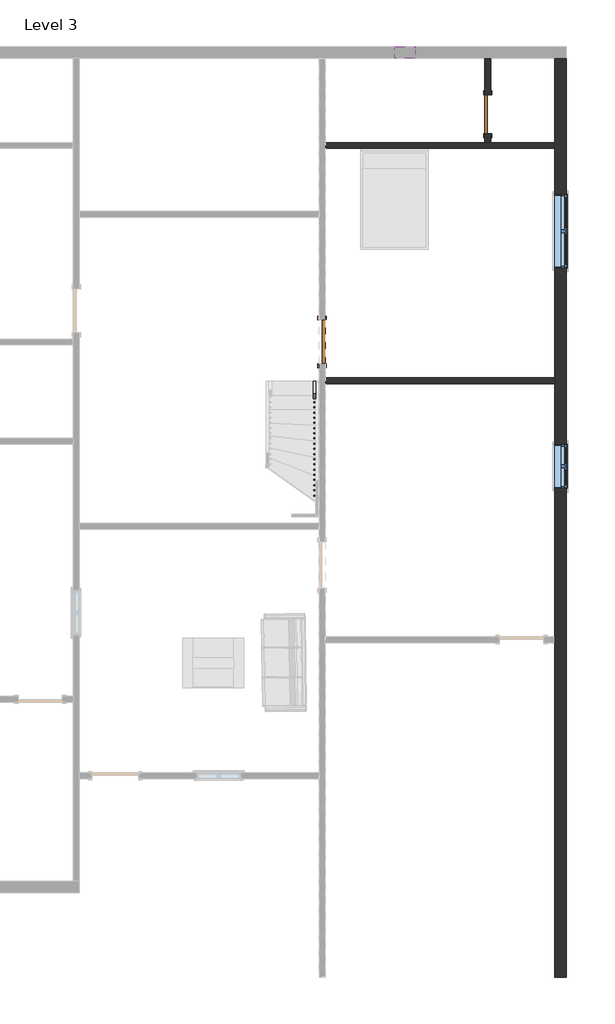
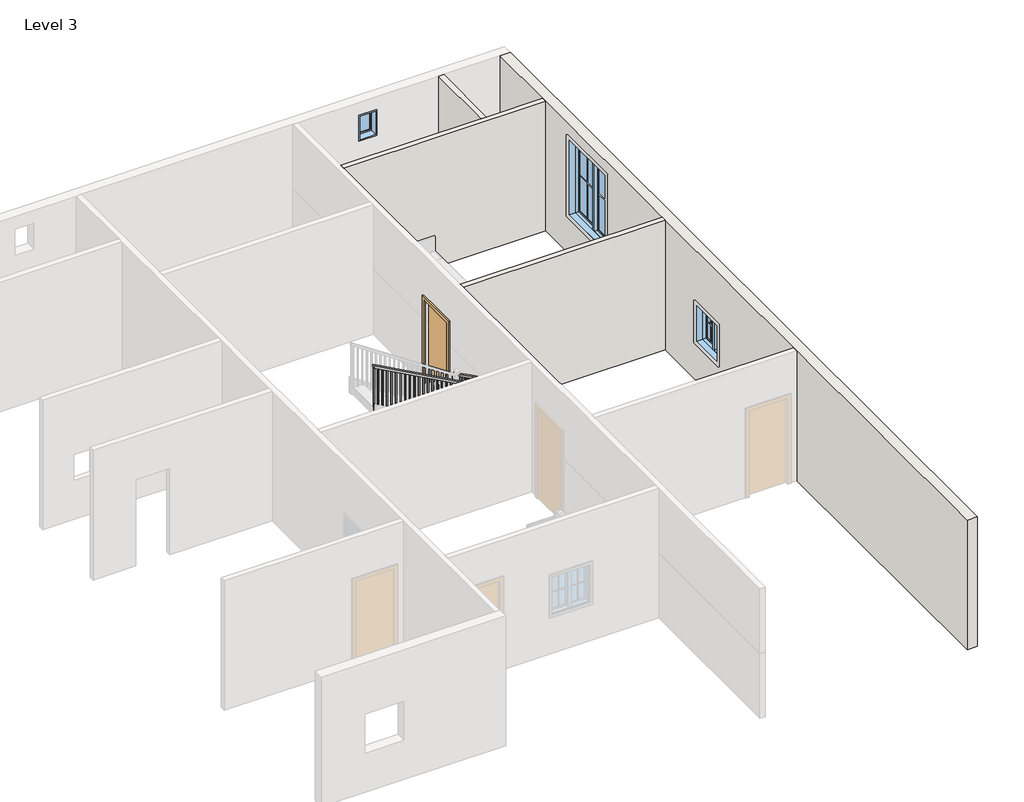
# One storey, part 2 of 3: 4 walls, 3 windows, 2 doors, 1 railing.
"""IFC4 building model written with IfcOpenShell, lengths in millimetres."""

from ifc_helpers import new_model, si_unit, frame, origin, place, context, project, spatial, polyline, outline, extrude, faceted_brep, transform, mapped, element, save
from components import door_f2b275c1, door_c29894e6, window_aa618e30, window_339605e1, window_9ac97e1a

model = new_model("IFC4")

# Units and contexts
model_context = context("Model", 3, world=origin())
ifc_project = project(units=[si_unit("LENGTHUNIT", "METRE", prefix="MILLI")], contexts=[model_context])

# Site, building, storey
site = spatial("IfcSite", under=ifc_project)
building = spatial("IfcBuilding", under=site)
storey = spatial("IfcBuildingStorey", under=building, Name="Level 3", Elevation=3200.4)

# Doors
placement = place(None, origin())
door_shape = door_f2b275c1(model_context)
element("IfcDoor", 1, ObjectType="Single-Flush : 30\" x 80\"", at=placement, inside=storey, context=model_context, shape_type="MappedRepresentation", body=[
    mapped(door_shape, transform((4827.3366507, 9100.7522623, 3200.4), x_axis=(0.0, -1.0, 0.0), y_axis=(1.0, 0.0, 0.0), z_axis=(0.0, 0.0, 1.0))),
])
door_2_shape = door_c29894e6(model_context)
element("IfcDoor", 2, ObjectType="Single-Flush : 34\" x 80\"", at=placement, inside=storey, context=model_context, shape_type="MappedRepresentation", body=[
    mapped(door_2_shape, transform((1583.2084916, 4643.0522623, 3200.4), x_axis=(0.0, -1.0, 0.0), y_axis=(1.0, 0.0, 0.0), z_axis=(0.0, 0.0, 1.0))),
])

# Railing
element("IfcRailing", 3, ObjectType="Handrail - Rectangular", at=placement, inside=storey, context=model_context, shape_type="SolidModel", body=[
    faceted_brep([(1456.2084916, 3870.4222402, 4284.1333333), (1456.2084916, 3870.4222402, 4227.1391458), (1405.4084916, 3870.4222402, 4227.1391458), (1405.4084916, 3870.4222402, 4284.1333333), (1456.2084916, 1506.6647172, 5486.478212), (1456.2084916, 1494.487215, 5435.678212), (1405.4084916, 1494.487215, 5435.678212), (1405.4084916, 1506.6647172, 5486.478212), (1456.2084916, 1268.9652728, 5486.478212), (1456.2084916, 1268.9652728, 5435.678212), (1405.4084916, 1319.7652728, 5435.678212), (1405.4084916, 1319.7652728, 5486.478212), (1234.4478889, 1268.9652728, 5486.478212), (1221.4006723, 1268.9652728, 5435.678212), (1221.4006723, 1319.7652728, 5435.678212), (1234.4478889, 1319.7652728, 5486.478212), (-1813.7050583, 1268.9652728, 7162.8), (-1813.7050583, 1319.7652728, 7162.8), (-1813.7050583, 1319.7652728, 7104.8247257), (-1813.7050583, 1268.9652728, 7104.8247257)], [[[0, 1, 2, 3]], [[1, 0, 4, 5]], [[2, 1, 5, 6]], [[3, 2, 6, 7]], [[0, 3, 7, 4]], [[5, 4, 8, 9]], [[6, 5, 9, 10]], [[7, 6, 10, 11]], [[4, 7, 11, 8]], [[9, 8, 12, 13]], [[10, 9, 13, 14]], [[11, 10, 14, 15]], [[8, 11, 15, 12]], [[16, 17, 18, 19]], [[13, 12, 16, 19]], [[14, 13, 19, 18]], [[15, 14, 18, 17]], [[12, 15, 17, 16]]]),
    extrude(outline(polyline([(7057.8655707, -1728.3165084), (6079.0666667, -1728.3165084), (6079.0666667, -1709.2665084), (7047.3890853, -1709.2665084), (7057.8655707, -1728.3165084)])), frame((0.0, 1284.8402728, 0.0), z_axis=(0.0, 1.0, 0.0), x_axis=(0.0, 0.0, 1.0)), (0.0, 0.0, 1.0), 19.05),
    extrude(outline(polyline([(7001.9909816, -1626.7165084), (6079.0666667, -1626.7165084), (6079.0666667, -1607.6665084), (6991.5144961, -1607.6665084), (7001.9909816, -1626.7165084)])), frame((0.0, 1284.8402728, 0.0), z_axis=(0.0, 1.0, 0.0), x_axis=(0.0, 0.0, 1.0)), (0.0, 0.0, 1.0), 19.05),
    extrude(outline(polyline([(6946.1163924, -1525.1165084), (5909.7333333, -1525.1165084), (5909.7333333, -1506.0665084), (6935.6399069, -1506.0665084), (6946.1163924, -1525.1165084)])), frame((0.0, 1284.8402728, 0.0), z_axis=(0.0, 1.0, 0.0), x_axis=(0.0, 0.0, 1.0)), (0.0, 0.0, 1.0), 19.05),
    extrude(outline(polyline([(6890.2418032, -1423.5165084), (5909.7333333, -1423.5165084), (5909.7333333, -1404.4665084), (6879.7653177, -1404.4665084), (6890.2418032, -1423.5165084)])), frame((0.0, 1284.8402728, 0.0), z_axis=(0.0, 1.0, 0.0), x_axis=(0.0, 0.0, 1.0)), (0.0, 0.0, 1.0), 19.05),
    extrude(outline(polyline([(6834.367214, -1321.9165084), (5909.7333333, -1321.9165084), (5909.7333333, -1302.8665084), (6823.8907286, -1302.8665084), (6834.367214, -1321.9165084)])), frame((0.0, 1284.8402728, 0.0), z_axis=(0.0, 1.0, 0.0), x_axis=(0.0, 0.0, 1.0)), (0.0, 0.0, 1.0), 19.05),
    extrude(outline(polyline([(6778.4926249, -1220.3165084), (5740.4, -1220.3165084), (5740.4, -1201.2665084), (6768.0161394, -1201.2665084), (6778.4926249, -1220.3165084)])), frame((0.0, 1284.8402728, 0.0), z_axis=(0.0, 1.0, 0.0), x_axis=(0.0, 0.0, 1.0)), (0.0, 0.0, 1.0), 19.05),
    extrude(outline(polyline([(6722.6180357, -1118.7165084), (5740.4, -1118.7165084), (5740.4, -1099.6665084), (6712.1415502, -1099.6665084), (6722.6180357, -1118.7165084)])), frame((0.0, 1284.8402728, 0.0), z_axis=(0.0, 1.0, 0.0), x_axis=(0.0, 0.0, 1.0)), (0.0, 0.0, 1.0), 19.05),
    extrude(outline(polyline([(6666.7434465, -1017.1165084), (5740.4, -1017.1165084), (5740.4, -998.0665084), (6656.266961, -998.0665084), (6666.7434465, -1017.1165084)])), frame((0.0, 1284.8402728, 0.0), z_axis=(0.0, 1.0, 0.0), x_axis=(0.0, 0.0, 1.0)), (0.0, 0.0, 1.0), 19.05),
    extrude(outline(polyline([(6610.8688573, -915.5165084), (5571.0666667, -915.5165084), (5571.0666667, -896.4665084), (6600.3923719, -896.4665084), (6610.8688573, -915.5165084)])), frame((0.0, 1284.8402728, 0.0), z_axis=(0.0, 1.0, 0.0), x_axis=(0.0, 0.0, 1.0)), (0.0, 0.0, 1.0), 19.05),
    extrude(outline(polyline([(6554.9942682, -813.9165084), (5571.0666667, -813.9165084), (5571.0666667, -794.8665084), (6544.5177827, -794.8665084), (6554.9942682, -813.9165084)])), frame((0.0, 1284.8402728, 0.0), z_axis=(0.0, 1.0, 0.0), x_axis=(0.0, 0.0, 1.0)), (0.0, 0.0, 1.0), 19.05),
    extrude(outline(polyline([(6499.119679, -712.3165084), (5571.0666667, -712.3165084), (5571.0666667, -693.2665084), (6488.6431935, -693.2665084), (6499.119679, -712.3165084)])), frame((0.0, 1284.8402728, 0.0), z_axis=(0.0, 1.0, 0.0), x_axis=(0.0, 0.0, 1.0)), (0.0, 0.0, 1.0), 19.05),
    extrude(outline(polyline([(6443.2450898, -610.7165084), (5401.7333333, -610.7165084), (5401.7333333, -591.6665084), (6432.7686044, -591.6665084), (6443.2450898, -610.7165084)])), frame((0.0, 1284.8402728, 0.0), z_axis=(0.0, 1.0, 0.0), x_axis=(0.0, 0.0, 1.0)), (0.0, 0.0, 1.0), 19.05),
    extrude(outline(polyline([(6387.3705007, -509.1165084), (5401.7333333, -509.1165084), (5401.7333333, -490.0665084), (6376.8940152, -490.0665084), (6387.3705007, -509.1165084)])), frame((0.0, 1284.8402728, 0.0), z_axis=(0.0, 1.0, 0.0), x_axis=(0.0, 0.0, 1.0)), (0.0, 0.0, 1.0), 19.05),
    extrude(outline(polyline([(6331.4959115, -407.5165084), (5401.7333333, -407.5165084), (5401.7333333, -388.4665084), (6321.019426, -388.4665084), (6331.4959115, -407.5165084)])), frame((0.0, 1284.8402728, 0.0), z_axis=(0.0, 1.0, 0.0), x_axis=(0.0, 0.0, 1.0)), (0.0, 0.0, 1.0), 19.05),
    extrude(outline(polyline([(6275.6213223, -305.9165084), (5232.4, -305.9165084), (5232.4, -286.8665084), (6265.1448368, -286.8665084), (6275.6213223, -305.9165084)])), frame((0.0, 1284.8402728, 0.0), z_axis=(0.0, 1.0, 0.0), x_axis=(0.0, 0.0, 1.0)), (0.0, 0.0, 1.0), 19.05),
    extrude(outline(polyline([(6219.7467331, -204.3165084), (5232.4, -204.3165084), (5232.4, -185.2665084), (6209.2702477, -185.2665084), (6219.7467331, -204.3165084)])), frame((0.0, 1284.8402728, 0.0), z_axis=(0.0, 1.0, 0.0), x_axis=(0.0, 0.0, 1.0)), (0.0, 0.0, 1.0), 19.05),
    extrude(outline(polyline([(6163.872144, -102.7165084), (5232.4, -102.7165084), (5232.4, -83.6665084), (6153.3956585, -83.6665084), (6163.872144, -102.7165084)])), frame((0.0, 1284.8402728, 0.0), z_axis=(0.0, 1.0, 0.0), x_axis=(0.0, 0.0, 1.0)), (0.0, 0.0, 1.0), 19.05),
    extrude(outline(polyline([(6107.9975548, -1.1165084), (5063.0666667, -1.1165084), (5063.0666667, 17.9334916), (6097.5210693, 17.9334916), (6107.9975548, -1.1165084)])), frame((0.0, 1284.8402728, 0.0), z_axis=(0.0, 1.0, 0.0), x_axis=(0.0, 0.0, 1.0)), (0.0, 0.0, 1.0), 19.05),
    extrude(outline(polyline([(6052.1229656, 100.4834916), (5063.0666667, 100.4834916), (5063.0666667, 119.5334916), (6041.6464801, 119.5334916), (6052.1229656, 100.4834916)])), frame((0.0, 1284.8402728, 0.0), z_axis=(0.0, 1.0, 0.0), x_axis=(0.0, 0.0, 1.0)), (0.0, 0.0, 1.0), 19.05),
    extrude(outline(polyline([(5996.2483764, 202.0834916), (5063.0666667, 202.0834916), (5063.0666667, 221.1334916), (5985.771891, 221.1334916), (5996.2483764, 202.0834916)])), frame((0.0, 1284.8402728, 0.0), z_axis=(0.0, 1.0, 0.0), x_axis=(0.0, 0.0, 1.0)), (0.0, 0.0, 1.0), 19.05),
    extrude(outline(polyline([(5940.3737873, 303.6834916), (4893.7333333, 303.6834916), (4893.7333333, 322.7334916), (5929.8973018, 322.7334916), (5940.3737873, 303.6834916)])), frame((0.0, 1284.8402728, 0.0), z_axis=(0.0, 1.0, 0.0), x_axis=(0.0, 0.0, 1.0)), (0.0, 0.0, 1.0), 19.05),
    extrude(outline(polyline([(5884.4991981, 405.2834916), (4893.7333333, 405.2834916), (4893.7333333, 424.3334916), (5874.0227126, 424.3334916), (5884.4991981, 405.2834916)])), frame((0.0, 1284.8402728, 0.0), z_axis=(0.0, 1.0, 0.0), x_axis=(0.0, 0.0, 1.0)), (0.0, 0.0, 1.0), 19.05),
    extrude(outline(polyline([(5828.6246089, 506.8834916), (4893.7333333, 506.8834916), (4893.7333333, 525.9334916), (5818.1481235, 525.9334916), (5828.6246089, 506.8834916)])), frame((0.0, 1284.8402728, 0.0), z_axis=(0.0, 1.0, 0.0), x_axis=(0.0, 0.0, 1.0)), (0.0, 0.0, 1.0), 19.05),
    extrude(outline(polyline([(5772.7500198, 608.4834916), (4724.4, 608.4834916), (4724.4, 627.5334916), (5762.2735343, 627.5334916), (5772.7500198, 608.4834916)])), frame((0.0, 1284.8402728, 0.0), z_axis=(0.0, 1.0, 0.0), x_axis=(0.0, 0.0, 1.0)), (0.0, 0.0, 1.0), 19.05),
    extrude(outline(polyline([(5716.8754306, 710.0834916), (4724.4, 710.0834916), (4724.4, 729.1334916), (5706.3989451, 729.1334916), (5716.8754306, 710.0834916)])), frame((0.0, 1284.8402728, 0.0), z_axis=(0.0, 1.0, 0.0), x_axis=(0.0, 0.0, 1.0)), (0.0, 0.0, 1.0), 19.05),
    extrude(outline(polyline([(5661.0008414, 811.6834916), (4724.4, 811.6834916), (4724.4, 830.7334916), (5650.5243559, 830.7334916), (5661.0008414, 811.6834916)])), frame((0.0, 1284.8402728, 0.0), z_axis=(0.0, 1.0, 0.0), x_axis=(0.0, 0.0, 1.0)), (0.0, 0.0, 1.0), 19.05),
    extrude(outline(polyline([(5605.1262522, 913.2834916), (4724.4, 913.2834916), (4724.4, 932.3334916), (5594.6497668, 932.3334916), (5605.1262522, 913.2834916)])), frame((0.0, 1284.8402728, 0.0), z_axis=(0.0, 1.0, 0.0), x_axis=(0.0, 0.0, 1.0)), (0.0, 0.0, 1.0), 19.05),
    extrude(outline(polyline([(5549.2516631, 1014.8834916), (4555.0666667, 1014.8834916), (4555.0666667, 1033.9334916), (5538.7751776, 1033.9334916), (5549.2516631, 1014.8834916)])), frame((0.0, 1284.8402728, 0.0), z_axis=(0.0, 1.0, 0.0), x_axis=(0.0, 0.0, 1.0)), (0.0, 0.0, 1.0), 19.05),
    extrude(outline(polyline([(5493.3770739, 1116.4834916), (4555.0666667, 1116.4834916), (4555.0666667, 1135.5334916), (5482.9005884, 1135.5334916), (5493.3770739, 1116.4834916)])), frame((0.0, 1284.8402728, 0.0), z_axis=(0.0, 1.0, 0.0), x_axis=(0.0, 0.0, 1.0)), (0.0, 0.0, 1.0), 19.05),
    extrude(outline(polyline([(5437.5024847, 1218.0834916), (4555.0666667, 1218.0834916), (4555.0666667, 1237.1334916), (5427.0259992, 1237.1334916), (5437.5024847, 1218.0834916)])), frame((0.0, 1284.8402728, 0.0), z_axis=(0.0, 1.0, 0.0), x_axis=(0.0, 0.0, 1.0)), (0.0, 0.0, 1.0), 19.05),
    extrude(outline(polyline([(1338.7334916, 1284.8402728), (1319.6834916, 1284.8402728), (1319.6834916, 1303.8902728), (1338.7334916, 1303.8902728), (1338.7334916, 1284.8402728)])), frame((0.0, 0.0, 4555.0666667), z_axis=(0.0, 0.0, 1.0), x_axis=(1.0, 0.0, 0.0)), (0.0, 0.0, 1.0), 880.6115453),
    extrude(outline(polyline([(1440.3334916, 1339.9472402), (1440.3334916, 1320.8972402), (1421.2834916, 1320.8972402), (1421.2834916, 1339.9472402), (1440.3334916, 1339.9472402)])), frame((0.0, 0.0, 4555.0666667), z_axis=(0.0, 0.0, 1.0), x_axis=(1.0, 0.0, 0.0)), (0.0, 0.0, 1.0), 880.6115453),
    extrude(outline(polyline([(1440.3334916, 1441.5472402), (1440.3334916, 1422.4972402), (1421.2834916, 1422.4972402), (1421.2834916, 1441.5472402), (1440.3334916, 1441.5472402)])), frame((0.0, 0.0, 4555.0666667), z_axis=(0.0, 0.0, 1.0), x_axis=(1.0, 0.0, 0.0)), (0.0, 0.0, 1.0), 880.6115453),
    extrude(outline(polyline([(1543.1472402, 5410.9268864), (1543.1472402, 4555.0666667), (1524.0972402, 4555.0666667), (1524.0972402, 5420.616827), (1543.1472402, 5410.9268864)])), frame((1421.2834916, 0.0, 0.0), z_axis=(1.0, 0.0, 0.0), x_axis=(0.0, 1.0, 0.0)), (0.0, 0.0, 1.0), 19.05),
    extrude(outline(polyline([(1644.7472402, 5359.2472033), (1644.7472402, 4385.7333333), (1625.6972402, 4385.7333333), (1625.6972402, 5368.9371439), (1644.7472402, 5359.2472033)])), frame((1421.2834916, 0.0, 0.0), z_axis=(1.0, 0.0, 0.0), x_axis=(0.0, 1.0, 0.0)), (0.0, 0.0, 1.0), 19.05),
    extrude(outline(polyline([(1746.3472402, 5307.5675203), (1746.3472402, 4385.7333333), (1727.2972402, 4385.7333333), (1727.2972402, 5317.2574608), (1746.3472402, 5307.5675203)])), frame((1421.2834916, 0.0, 0.0), z_axis=(1.0, 0.0, 0.0), x_axis=(0.0, 1.0, 0.0)), (0.0, 0.0, 1.0), 19.05),
    extrude(outline(polyline([(1847.9472402, 5255.8878372), (1847.9472402, 4385.7333333), (1828.8972402, 4385.7333333), (1828.8972402, 5265.5777778), (1847.9472402, 5255.8878372)])), frame((1421.2834916, 0.0, 0.0), z_axis=(1.0, 0.0, 0.0), x_axis=(0.0, 1.0, 0.0)), (0.0, 0.0, 1.0), 19.05),
    extrude(outline(polyline([(1949.5472402, 5204.2081541), (1949.5472402, 4385.7333333), (1930.4972402, 4385.7333333), (1930.4972402, 5213.8980947), (1949.5472402, 5204.2081541)])), frame((1421.2834916, 0.0, 0.0), z_axis=(1.0, 0.0, 0.0), x_axis=(0.0, 1.0, 0.0)), (0.0, 0.0, 1.0), 19.05),
    extrude(outline(polyline([(2051.1472402, 5152.528471), (2051.1472402, 4216.4), (2032.0972402, 4216.4), (2032.0972402, 5162.2184116), (2051.1472402, 5152.528471)])), frame((1421.2834916, 0.0, 0.0), z_axis=(1.0, 0.0, 0.0), x_axis=(0.0, 1.0, 0.0)), (0.0, 0.0, 1.0), 19.05),
    extrude(outline(polyline([(2152.7472402, 5100.8487879), (2152.7472402, 4216.4), (2133.6972402, 4216.4), (2133.6972402, 5110.5387285), (2152.7472402, 5100.8487879)])), frame((1421.2834916, 0.0, 0.0), z_axis=(1.0, 0.0, 0.0), x_axis=(0.0, 1.0, 0.0)), (0.0, 0.0, 1.0), 19.05),
    extrude(outline(polyline([(2254.3472402, 5049.1691048), (2254.3472402, 4216.4), (2235.2972402, 4216.4), (2235.2972402, 5058.8590454), (2254.3472402, 5049.1691048)])), frame((1421.2834916, 0.0, 0.0), z_axis=(1.0, 0.0, 0.0), x_axis=(0.0, 1.0, 0.0)), (0.0, 0.0, 1.0), 19.05),
    extrude(outline(polyline([(2355.9472402, 4997.4894218), (2355.9472402, 4216.4), (2336.8972402, 4216.4), (2336.8972402, 5007.1793623), (2355.9472402, 4997.4894218)])), frame((1421.2834916, 0.0, 0.0), z_axis=(1.0, 0.0, 0.0), x_axis=(0.0, 1.0, 0.0)), (0.0, 0.0, 1.0), 19.05),
    extrude(outline(polyline([(2457.5472402, 4945.8097387), (2457.5472402, 4047.0666667), (2438.4972402, 4047.0666667), (2438.4972402, 4955.4996793), (2457.5472402, 4945.8097387)])), frame((1421.2834916, 0.0, 0.0), z_axis=(1.0, 0.0, 0.0), x_axis=(0.0, 1.0, 0.0)), (0.0, 0.0, 1.0), 19.05),
    extrude(outline(polyline([(2559.1472402, 4894.1300556), (2559.1472402, 4047.0666667), (2540.0972402, 4047.0666667), (2540.0972402, 4903.8199962), (2559.1472402, 4894.1300556)])), frame((1421.2834916, 0.0, 0.0), z_axis=(1.0, 0.0, 0.0), x_axis=(0.0, 1.0, 0.0)), (0.0, 0.0, 1.0), 19.05),
    extrude(outline(polyline([(2660.7472402, 4842.4503725), (2660.7472402, 4047.0666667), (2641.6972402, 4047.0666667), (2641.6972402, 4852.1403131), (2660.7472402, 4842.4503725)])), frame((1421.2834916, 0.0, 0.0), z_axis=(1.0, 0.0, 0.0), x_axis=(0.0, 1.0, 0.0)), (0.0, 0.0, 1.0), 19.05),
    extrude(outline(polyline([(2762.3472402, 4790.7706894), (2762.3472402, 3877.7333333), (2743.2972402, 3877.7333333), (2743.2972402, 4800.46063), (2762.3472402, 4790.7706894)])), frame((1421.2834916, 0.0, 0.0), z_axis=(1.0, 0.0, 0.0), x_axis=(0.0, 1.0, 0.0)), (0.0, 0.0, 1.0), 19.05),
    extrude(outline(polyline([(2863.9472402, 4739.0910064), (2863.9472402, 3877.7333333), (2844.8972402, 3877.7333333), (2844.8972402, 4748.7809469), (2863.9472402, 4739.0910064)])), frame((1421.2834916, 0.0, 0.0), z_axis=(1.0, 0.0, 0.0), x_axis=(0.0, 1.0, 0.0)), (0.0, 0.0, 1.0), 19.05),
    extrude(outline(polyline([(2965.5472402, 4687.4113233), (2965.5472402, 3877.7333333), (2946.4972402, 3877.7333333), (2946.4972402, 4697.1012638), (2965.5472402, 4687.4113233)])), frame((1421.2834916, 0.0, 0.0), z_axis=(1.0, 0.0, 0.0), x_axis=(0.0, 1.0, 0.0)), (0.0, 0.0, 1.0), 19.05),
    extrude(outline(polyline([(3067.1472402, 4635.7316402), (3067.1472402, 3708.4), (3048.0972402, 3708.4), (3048.0972402, 4645.4215808), (3067.1472402, 4635.7316402)])), frame((1421.2834916, 0.0, 0.0), z_axis=(1.0, 0.0, 0.0), x_axis=(0.0, 1.0, 0.0)), (0.0, 0.0, 1.0), 19.05),
    extrude(outline(polyline([(3168.7472402, 4584.0519571), (3168.7472402, 3708.4), (3149.6972402, 3708.4), (3149.6972402, 4593.7418977), (3168.7472402, 4584.0519571)])), frame((1421.2834916, 0.0, 0.0), z_axis=(1.0, 0.0, 0.0), x_axis=(0.0, 1.0, 0.0)), (0.0, 0.0, 1.0), 19.05),
    extrude(outline(polyline([(3270.3472402, 4532.372274), (3270.3472402, 3708.4), (3251.2972402, 3708.4), (3251.2972402, 4542.0622146), (3270.3472402, 4532.372274)])), frame((1421.2834916, 0.0, 0.0), z_axis=(1.0, 0.0, 0.0), x_axis=(0.0, 1.0, 0.0)), (0.0, 0.0, 1.0), 19.05),
    extrude(outline(polyline([(3371.9472402, 4480.6925909), (3371.9472402, 3539.0666667), (3352.8972402, 3539.0666667), (3352.8972402, 4490.3825315), (3371.9472402, 4480.6925909)])), frame((1421.2834916, 0.0, 0.0), z_axis=(1.0, 0.0, 0.0), x_axis=(0.0, 1.0, 0.0)), (0.0, 0.0, 1.0), 19.05),
    extrude(outline(polyline([(3473.5472402, 4429.0129079), (3473.5472402, 3539.0666667), (3454.4972402, 3539.0666667), (3454.4972402, 4438.7028484), (3473.5472402, 4429.0129079)])), frame((1421.2834916, 0.0, 0.0), z_axis=(1.0, 0.0, 0.0), x_axis=(0.0, 1.0, 0.0)), (0.0, 0.0, 1.0), 19.05),
    extrude(outline(polyline([(3575.1472402, 4377.3332248), (3575.1472402, 3539.0666667), (3556.0972402, 3539.0666667), (3556.0972402, 4387.0231654), (3575.1472402, 4377.3332248)])), frame((1421.2834916, 0.0, 0.0), z_axis=(1.0, 0.0, 0.0), x_axis=(0.0, 1.0, 0.0)), (0.0, 0.0, 1.0), 19.05),
    extrude(outline(polyline([(3676.7472402, 4325.6535417), (3676.7472402, 3369.7333333), (3657.6972402, 3369.7333333), (3657.6972402, 4335.3434823), (3676.7472402, 4325.6535417)])), frame((1421.2834916, 0.0, 0.0), z_axis=(1.0, 0.0, 0.0), x_axis=(0.0, 1.0, 0.0)), (0.0, 0.0, 1.0), 19.05),
    extrude(outline(polyline([(3778.3472402, 4273.9738586), (3778.3472402, 3369.7333333), (3759.2972402, 3369.7333333), (3759.2972402, 4283.6637992), (3778.3472402, 4273.9738586)])), frame((1421.2834916, 0.0, 0.0), z_axis=(1.0, 0.0, 0.0), x_axis=(0.0, 1.0, 0.0)), (0.0, 0.0, 1.0), 19.05),
    extrude(outline(polyline([(1440.3334916, 1303.8902728), (1440.3334916, 1284.8402728), (1421.2834916, 1284.8402728), (1421.2834916, 1303.8902728), (1440.3334916, 1303.8902728)])), frame((0.0, 0.0, 4555.0666667), z_axis=(0.0, 0.0, 1.0), x_axis=(1.0, 0.0, 0.0)), (0.0, 0.0, 1.0), 880.6115453),
    extrude(outline(polyline([(7104.8247257, -1813.7050583), (6079.0666667, -1813.7050583), (6079.0666667, -1794.6550583), (7094.3482402, -1794.6550583), (7104.8247257, -1813.7050583)])), frame((0.0, 1284.8402728, 0.0), z_axis=(0.0, 1.0, 0.0), x_axis=(0.0, 0.0, 1.0)), (0.0, 0.0, 1.0), 19.05),
    extrude(outline(polyline([(3870.4222402, 4227.1391458), (3870.4222402, 3369.7333333), (3851.3722402, 3369.7333333), (3851.3722402, 4236.8290864), (3870.4222402, 4227.1391458)])), frame((1421.2834916, 0.0, 0.0), z_axis=(1.0, 0.0, 0.0), x_axis=(0.0, 1.0, 0.0)), (0.0, 0.0, 1.0), 19.05),
])

# Walls
element("IfcWall", 4, ObjectType="9\"", at=placement, inside=storey, context=model_context, shape_type="Brep", body=[
    faceted_brep([(6136.1584916, 10199.3022623, 3200.4), (6136.1584916, 8548.3022623, 3200.4), (6136.1584916, 8434.0022623, 3200.4), (6136.1584916, 3938.2022623, 3200.4), (6136.1584916, 3823.9022623, 3200.4), (6136.1584916, -1129.0977377, 3200.4), (6136.1584916, -1243.3977377, 3200.4), (6136.1584916, -7802.9477377, 3200.4), (6136.1584916, -7802.9477377, 6248.4), (6136.1584916, -1243.3977377, 6248.4), (6136.1584916, -1129.0977377, 6248.4), (6136.1584916, 3823.9022623, 6248.4), (6136.1584916, 3938.2022623, 6248.4), (6136.1584916, 8434.0022623, 6248.4), (6136.1584916, 8548.3022623, 6248.4), (6136.1584916, 10199.3022623, 6248.4), (6136.1584916, 1772.8522623, 5029.2), (6136.1584916, 1772.8522623, 4114.8), (6136.1584916, 2636.4522623, 4114.8), (6136.1584916, 2636.4522623, 5029.2), (6136.1584916, 6090.8522623, 5943.6), (6136.1584916, 6090.8522623, 4114.8), (6136.1584916, 7538.6522623, 4114.8), (6136.1584916, 7538.6522623, 5943.6), (6364.7584916, 10199.3022623, 3200.4), (6364.7584916, 10199.3022623, 6248.4), (6364.7584916, -7802.9477377, 6248.4), (6364.7584916, -7802.9477377, 3200.4), (6364.7584916, 1772.8522623, 5029.2), (6364.7584916, 2636.4522623, 5029.2), (6364.7584916, 2636.4522623, 4114.8), (6364.7584916, 1772.8522623, 4114.8), (6364.7584916, 6090.8522623, 5943.6), (6364.7584916, 7538.6522623, 5943.6), (6364.7584916, 7538.6522623, 4114.8), (6364.7584916, 6090.8522623, 4114.8)], [[[0, 1, 2, 3, 4, 5, 6, 7, 8, 9, 10, 11, 12, 13, 14, 15], [16, 17, 18, 19], [20, 21, 22, 23]], [[24, 25, 26, 27], [28, 29, 30, 31], [32, 33, 34, 35]], [[7, 6, 5, 4, 3, 2, 1, 0, 24, 27]], [[8, 7, 27, 26]], [[0, 15, 25, 24]], [[17, 16, 28, 31]], [[18, 17, 31, 30]], [[19, 18, 30, 29]], [[16, 19, 29, 28]], [[21, 20, 32, 35]], [[22, 21, 35, 34]], [[23, 22, 34, 33]], [[20, 23, 33, 32]], [[15, 14, 13, 12, 11, 10, 9, 8, 26, 25]]]),
])
element("IfcWall", 5, ObjectType="WALL4.5\"", at=placement, inside=storey, context=model_context, shape_type="SweptSolid", body=[
    extrude(outline(polyline([(8719.7522623, 5232.4), (8719.7522623, 3200.4), (8548.3022623, 3200.4), (8548.3022623, 6248.4), (10199.3022623, 6248.4), (10199.3022623, 3200.4), (9481.7522623, 3200.4), (9481.7522623, 5232.4), (8719.7522623, 5232.4)])), frame((4770.1866507, 0.0, 0.0), z_axis=(1.0, 0.0, 0.0), x_axis=(0.0, 1.0, 0.0)), (0.0, 0.0, 1.0), 114.3),
])
element("IfcWall", 6, ObjectType="WALL4.5\"", at=placement, inside=storey, context=model_context, shape_type="Brep", body=[
    faceted_brep([(1640.3584916, 8434.0022623, 6248.4), (1640.3584916, 8434.0022623, 3200.4), (6136.1584916, 8434.0022623, 3200.4), (6136.1584916, 8434.0022623, 6248.4), (1640.3584916, 8548.3022623, 3200.4), (1640.3584916, 8548.3022623, 6248.4), (4770.1866507, 8548.3022623, 6248.4), (4884.4866507, 8548.3022623, 6248.4), (6136.1584916, 8548.3022623, 6248.4), (6136.1584916, 8548.3022623, 3200.4), (4884.4866507, 8548.3022623, 3200.4), (4770.1866507, 8548.3022623, 3200.4)], [[[0, 1, 2, 3]], [[4, 5, 6, 7, 8, 9, 10, 11]], [[2, 1, 4, 11, 10, 9]], [[3, 2, 9, 8]], [[0, 3, 8, 7, 6, 5]], [[0, 5, 4, 1]]]),
])
element("IfcWall", 7, ObjectType="WALL4.5\"", at=placement, inside=storey, context=model_context, shape_type="SweptSolid", body=[
    extrude(outline(polyline([(6136.1584916, 3823.9022623), (1640.3584916, 3823.9022623), (1640.3584916, 3938.2022623), (6136.1584916, 3938.2022623), (6136.1584916, 3823.9022623)])), frame((0.0, 0.0, 3200.4), z_axis=(0.0, 0.0, 1.0), x_axis=(1.0, 0.0, 0.0)), (0.0, 0.0, 1.0), 3048.0),
])

# Windows
window_shape = window_aa618e30(model_context)
element("IfcWindow", 8, ObjectType="Fixed : 16\" x 24\"", at=placement, inside=storey, context=model_context, shape_type="MappedRepresentation", body=[
    mapped(window_shape, transform((3243.3725711, 10313.6022623, 4419.6), x_axis=(1.0, 0.0, 0.0), y_axis=(0.0, 1.0, 0.0), z_axis=(0.0, 0.0, 1.0))),
])
window_2_shape = window_339605e1(model_context)
element("IfcWindow", 9, ObjectType="Window-Casement-Double : 34\" x 36\"", at=placement, inside=storey, context=model_context, shape_type="MappedRepresentation", body=[
    mapped(window_2_shape, transform((6250.4584916, 2204.6522623, 3200.4), x_axis=(0.0, -1.0, 0.0), y_axis=(1.0, 0.0, 0.0), z_axis=(0.0, 0.0, 1.0))),
])
window_3_shape = window_9ac97e1a(model_context)
element("IfcWindow", 10, ObjectType="Window-Casement-Double : 57\" x 72\"", at=placement, inside=storey, context=model_context, shape_type="MappedRepresentation", body=[
    mapped(window_3_shape, transform((6250.4584916, 6814.7522623, 3200.4), x_axis=(0.0, -1.0, 0.0), y_axis=(1.0, 0.0, 0.0), z_axis=(0.0, 0.0, 1.0))),
])

save(model, "model.ifc")

# Revit data of these elements
# Type "Single-Flush : 30\" x 80\""
#   Type Mark = "5"
#   Construction Type Id = "MDOOR"
#   Assembly Code = "C1020"
#   Analytic Construction = "Metal"
#   Thickness = 0' - 2"
#   Heat Transfer Coefficient (U) = 0.651978 BTU/(h·ft²·°F)
#   Height = 6' - 8"
#   Trim Projection Ext = 0' - 1"
#   Trim Projection Int = 0' - 1"
#   Trim Width = 0' - 3"
#   Width = 2' - 6"
#   Define Thermal Properties by = 1
#   Define Thermal Properties by = 1
#   Door Material = Door - Panel
#   Frame Material = Door - Frame
#   Visual Light Transmittance = 0
#   Solar Heat Gain Coefficient = 0
#   Function = (empty or 0)
#   Wall Closure = (empty or 0)
# Type "Single-Flush : 34\" x 80\""
#   Type Mark = "7"
#   Construction Type Id = "MDOOR"
#   Assembly Code = "C1020"
#   Analytic Construction = "Metal"
#   Thickness = 0' - 2"
#   Heat Transfer Coefficient (U) = 0.651978 BTU/(h·ft²·°F)
#   Height = 6' - 8"
#   Trim Projection Ext = 0' - 1"
#   Trim Projection Int = 0' - 1"
#   Trim Width = 0' - 3"
#   Width = 2' - 10"
#   Define Thermal Properties by = 1
#   Define Thermal Properties by = 1
#   Door Material = Door - Panel
#   Frame Material = Door - Frame
#   Visual Light Transmittance = 0
#   Solar Heat Gain Coefficient = 0
#   Function = (empty or 0)
#   Wall Closure = (empty or 0)
# Type "Handrail - Rectangular"
#   Assembly Code = "C2010400"
#   built-in parameter 1008612 = 0.0416667 (stored number, unit not read)
#   built-in parameter 1008611 = 0.0416667 (stored number, unit not read)
#   built-in parameter 1008609 = 0.333333 (stored number, unit not read)
#   built-in parameter 1008604 = 0.166667 (stored number, unit not read)
#   built-in parameter 1008603 = 0.166667 (stored number, unit not read)
#   Railing Height = 3' - 0"
#   built-in parameter 1008630 = 2
#   built-in parameter 1008610 = 2
#   built-in parameter 1008618 = Baluster - Square : 3/4"
# Type "9\""
#   Assembly Code = "B2010"
#   Layers, outside or top first: 0' - 9" no material (function 1)
# Type "WALL4.5\""
#   Assembly Code = "B2010"
#   Layers, outside or top first: 0' - 4 1/2" no material (function 1)
# Type "Fixed : 16\" x 24\""
#   Type Mark = "4"
#   Construction Type Id = "GSP4R"
#   Assembly Code = "B2020100"
#   Analytic Construction = "1/8 in Pilkington single glazing"
#   Visual Light Transmittance = 0.9
#   Solar Heat Gain Coefficient = 0.78
#   Heat Transfer Coefficient (U) = 0.6496 BTU/(h·ft²·°F)
#   Height = 2' - 0"
#   Default Sill Height = 3' - 0"
#   Width = 1' - 4"
#   Window Inset = 0' - 0 3/4"
#   Define Thermal Properties by = 1
#   Define Thermal Properties by = 1
#   Glass Pane Material = Glass
#   Sash Material = Sash
#   Wall Closure = (empty or 0)
# Type "Window-Casement-Double : 34\" x 36\""
#   Type Mark = "14"
#   Fire Rating = "0.5h"
#   Assembly Code = "B2020100"
#   Analytic Construction = "Double glazing - domestic"
#   Frame Extension [instance default] = 0' - 0 1/4"
#   Window Inset [instance default] = 0' - 0"
#   Wall Thickness [instance default] = 0' - 6"
#   Interior Wall Closure [instance default] = 0' - 2 1/4"
#   Half Width = 1' - 5"
#   Visual Light Transmittance = 0.81
#   Thermal Resistance (R) = 1.8146 (h·ft²·°F)/BTU
#   Solar Heat Gain Coefficient = 0.76
#   Rough Width = 2' - 10 1/2"
#   Rough Height = 3' - 0 1/2"
#   Height = 3' - 0"
#   Heat Transfer Coefficient (U) = 0.5511 BTU/(h·ft²·°F)
#   Exterior Wall Closure [instance default] = 0' - 1 1/4"
#   Extension Jamb [instance default] = 0' - 2 1/4"
#   Default Sill Height = 3' - 0"
#   Width = 2' - 10"
#   Define Thermal Properties by = 0
#   Muntin Visibility = yes
#   Interior Trim Visibility [instance default] = yes
#   Exterior Trim Visibility [instance default] = yes
#   Extension Jamb Visibility [instance default] = yes
#   Interior Trim Material = Wood - Stained
#   Muntin Pattern = Muntin Pattern_2x2 : Muntin Pattern_2x2
#   Interior Trim = Trim-Window-Interior-Flat : Picture Frame
#   Interior Frame Material = Wood - Stained
#   Glass Panel Material = Glass
#   Exterior Trim Material = Clad - White
#   Exterior Trim = Trim-Window-Exterior-Flat : with Sill
#   Exterior Frame Material = Clad - White
#   Wall Closure = (empty or 0)
# Type "Window-Casement-Double : 57\" x 72\""
#   Type Mark = "17"
#   Fire Rating = "0.5h"
#   Assembly Code = "B2020100"
#   Analytic Construction = "Double glazing - domestic"
#   Frame Extension [instance default] = 0' - 0 1/4"
#   Window Inset [instance default] = 0' - 0"
#   Wall Thickness [instance default] = 0' - 6"
#   Interior Wall Closure [instance default] = 0' - 2 1/4"
#   Half Width = 2' - 4 1/2"
#   Visual Light Transmittance = 0.81
#   Thermal Resistance (R) = 1.8146 (h·ft²·°F)/BTU
#   Solar Heat Gain Coefficient = 0.76
#   Rough Width = 4' - 9 1/2"
#   Rough Height = 6' - 0 1/2"
#   Height = 6' - 0"
#   Heat Transfer Coefficient (U) = 0.5511 BTU/(h·ft²·°F)
#   Exterior Wall Closure [instance default] = 0' - 1 1/4"
#   Extension Jamb [instance default] = 0' - 2 1/4"
#   Default Sill Height = 3' - 0"
#   Width = 4' - 9"
#   Define Thermal Properties by = 0
#   Muntin Visibility = yes
#   Interior Trim Visibility [instance default] = yes
#   Exterior Trim Visibility [instance default] = yes
#   Extension Jamb Visibility [instance default] = yes
#   Interior Trim Material = Wood - Stained
#   Muntin Pattern = Muntin Pattern_2x2 : Muntin Pattern_2x2
#   Interior Trim = Trim-Window-Interior-Flat : Picture Frame
#   Interior Frame Material = Wood - Stained
#   Glass Panel Material = Glass
#   Exterior Trim Material = Clad - White
#   Exterior Trim = Trim-Window-Exterior-Flat : with Sill
#   Exterior Frame Material = Clad - White
#   Wall Closure = (empty or 0)
# Element 1 (IfcDoor, "Single-Flush : 30\" x 80\"")
#   Phase Created = New Construction
#   Materials on its faces: "Door - Frame", "Door - Panel"
# Element 2 (IfcDoor, "Single-Flush : 34\" x 80\"")
#   Phase Created = New Construction
#   Materials on its faces: "Door - Frame", "Door - Panel"
# Element 3 (IfcRailing, "Handrail - Rectangular")
#   Phase Created = New Construction
# Element 4 (IfcWall, "9\"")
#   Top Offset = 0' - 0"
#   Base Offset = 0' - 0"
#   Unconnected Height = 10' - 0"
#   wall height = 10' - 0"
#   Phase Created = New Construction
#   Base Constraint = Level 3
#   Materials on its faces: "Default Wall", "legs"
# Elements 5, 6, 7 (IfcWall, "WALL4.5\"")
#   Top Offset = 0' - 0"
#   Base Offset = 0' - 0"
#   Unconnected Height = 10' - 0"
#   wall height = 10' - 0"
#   Phase Created = New Construction
#   Base Constraint = Level 3
#   Materials on its faces: "Default Wall"
# Element 8 (IfcWindow, "Fixed : 16\" x 24\"")
#   Mark = "12"
#   Phase Created = New Construction
#   Materials on its faces: "Sash", "Glass"
# Element 9 (IfcWindow, "Window-Casement-Double : 34\" x 36\"")
#   Mark = "18"
#   Window Inset = 0' - 0"
#   Interior Wall Closure = 0' - 2 1/4"
#   Frame Extension = 0' - 0 1/4"
#   Exterior Wall Closure = 0' - 1 1/4"
#   Interior Trim Visibility = yes
#   Exterior Trim Visibility = yes
#   Phase Created = New Construction
#   Materials on its faces: "Wood - Stained", "Glass", "Clad - White"
# Element 10 (IfcWindow, "Window-Casement-Double : 57\" x 72\"")
#   Mark = "19"
#   Window Inset = 0' - 0"
#   Interior Wall Closure = 0' - 2 1/4"
#   Frame Extension = 0' - 0 1/4"
#   Exterior Wall Closure = 0' - 1 1/4"
#   Interior Trim Visibility = yes
#   Exterior Trim Visibility = yes
#   Phase Created = New Construction
#   Materials on its faces: "Wood - Stained", "Glass", "Clad - White"
# Materials
#   "Door - Panel": class "Wood", colour RGB 210 159 95, transparency 0, Cost = 0
#   "Door - Frame": colour RGB 118 70 51, transparency 0, Cost = 0
#   "Glass": class "Glass", colour RGB 0 128 192, transparency 0.75, Description = "Soda Lime Glass", Cost = 0
#   "Sash": class "Wood", colour RGB 224 178 126, transparency 0, Cost = 0
#   "Wood - Stained": class "Wood", colour RGB 224 178 126, transparency 0, Cost = 0
#   "Clad - White": class "Wood", colour RGB 242 242 238, transparency 0, Cost = 0
#   "Default Wall": colour RGB 128 128 128, transparency 0, Cost = 0
#   "legs": colour RGB 90 73 37, transparency 0, Cost = 0
